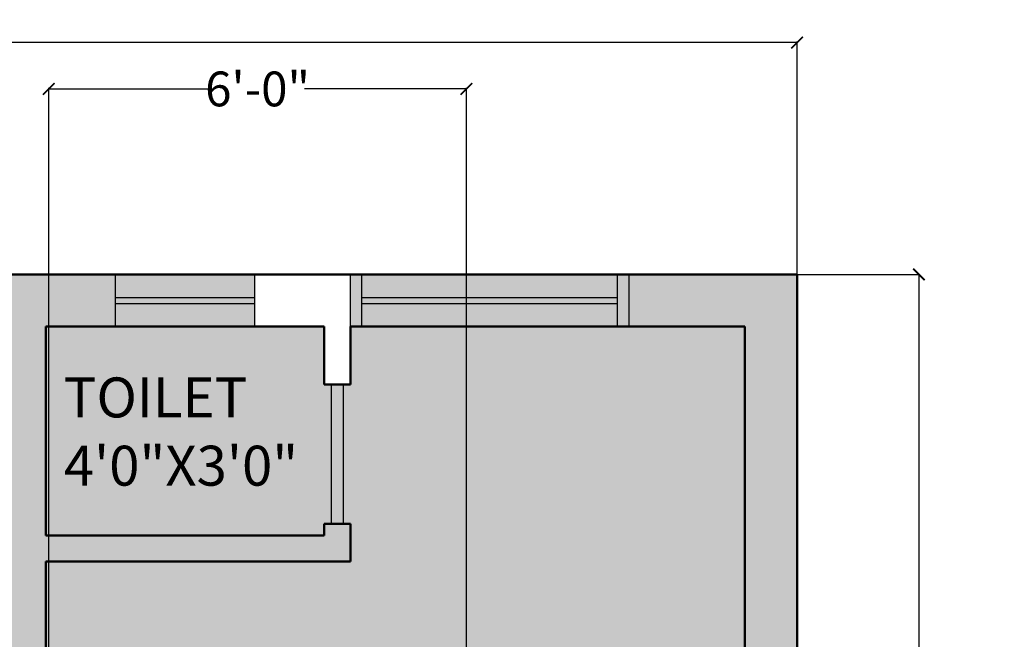
# Model space of a CAD drawing. Units: inches. Extents: x 528 to 2620, y -1066 to 798.
# Tile 34 of 41: x 1211 to 1381, y 656 to 763. Entities that reach past the tile are written whole.
import ezdxf

# ---------------------------------------------------------------- set-up
doc = ezdxf.new("R2010")
doc.units = ezdxf.units.IN
doc.header["$MEASUREMENT"] = 0
for name, color, linetype, lineweight in [('A-ANNO-DIMS', 2, 'Continuous', 18), ('A-AREA-IDEN', 7, 'Continuous', 18), ('A-Door', 2, 'Continuous', 25), ('A-GLAZ', 3, 'Continuous', 25), ('A-WALL', 7, 'Continuous', 50), ('A-WALL-PATT', 8, 'Continuous', 13)]:
    doc.layers.add(name, color=color, linetype=linetype, lineweight=lineweight)
doc.styles.get("Standard").update_dxf_attribs({"font": 'arial.ttf'})
doc.dimstyles.get("Standard").update_dxf_attribs({"dimtxt": 6, "dimasz": 2, "dimexe": 0.18, "dimexo": 0.0625, "dimgap": 0.09, "dimtad": 0, "dimtih": 1, "dimtoh": 1, "dimdec": 1, "dimzin": 0, "dimdsep": 46, "dimlunit": 3, "dimtxsty": 'Standard', "dimblk": 'ARCHTICK', "dimcen": 0.09, "dimadec": 0, "dimazin": 0, "dimtfac": 1, "dimtdec": 1, "dimtofl": 0, "dimtmove": 0, "dimatfit": 3, "dimfxl": 1, "dimtolj": 1, "dimtzin": 0, "dimarcsym": 0})

# ---------------------------------------------------------------- blocks, each defined once
blk = doc.blocks.new('_ArchTick')
at = {"color": 0, "linetype": 'ByBlock', "const_width": 0.15}
blk.add_lwpolyline([(-0.5, -0.5), (0.5, 0.5)], dxfattribs=at)
blk = doc.blocks.new('*D17')
at = {"layer": 'A-ANNO-DIMS', "color": 0, "lineweight": -2, "transparency": 16777216}
for p, q in [((1345.06, 718.92), (1366.18, 718.92)), ((1366, 718.92), (1366, 497.08)), ((1366, 268.92), (1366, 490.77)), ((1345.06, 268.92), (1366.18, 268.92))]:
    blk.add_line(p, q, dxfattribs=at)
at = {"layer": 'Defpoints', "color": 0, "transparency": 16777216}
for p in [(1345, 718.92), (1345, 268.92), (1366, 268.92)]:
    blk.add_point(p, dxfattribs=at)
at = {"layer": 'A-ANNO-DIMS', "color": 0, "lineweight": -2, "transparency": 16777216, "xscale": 2, "yscale": 2, "zscale": 2}
for p, rotation in [((1366, 718.92), 90), ((1366, 268.92), 270)]:
    blk.add_blockref('_ArchTick', p, dxfattribs=dict(at, rotation=rotation))
at = {"layer": 'A-ANNO-DIMS', "color": 0, "transparency": 16777216, "insert": (1366, 493.92), "char_height": 6, "attachment_point": 5}
blk.add_mtext('\\A1;37\'-6.0"', dxfattribs=at)
blk = doc.blocks.new('*D18')
at = {"layer": 'A-ANNO-DIMS', "color": 0, "lineweight": -2, "transparency": 16777216}
for p, q in [((1057, 718.98), (1057, 759.11)), ((1057, 758.93), (1195.76, 758.93)), ((1345, 758.93), (1206.23, 758.93)), ((1345, 718.98), (1345, 759.11))]:
    blk.add_line(p, q, dxfattribs=at)
at = {"layer": 'Defpoints', "color": 0, "transparency": 16777216}
for p in [(1345, 758.93), (1057, 718.92), (1345, 718.92)]:
    blk.add_point(p, dxfattribs=at)
at = {"layer": 'A-ANNO-DIMS', "color": 0, "lineweight": -2, "transparency": 16777216, "xscale": 2, "yscale": 2, "zscale": 2, "rotation": 180}
blk.add_blockref('_ArchTick', (1057, 758.93), dxfattribs=at)
at = {"layer": 'A-ANNO-DIMS', "color": 0, "lineweight": -2, "transparency": 16777216, "xscale": 2, "yscale": 2, "zscale": 2}
blk.add_blockref('_ArchTick', (1345, 758.93), dxfattribs=at)
at = {"layer": 'A-ANNO-DIMS', "color": 0, "transparency": 16777216, "insert": (1201, 758.93), "char_height": 6, "attachment_point": 5}
blk.add_mtext("\\A1;24'", dxfattribs=at)
blk = doc.blocks.new('WIN-1200')
for p, q in [((677.56, 718.92), (725.56, 718.92)), ((677.56, 709.92), (677.56, 718.92)), ((679.56, 709.92), (679.56, 718.92)), ((723.56, 718.92), (723.56, 709.92)), ((725.56, 718.92), (725.56, 709.92)), ((679.56, 714.92), (723.56, 714.92)), ((679.56, 713.92), (723.56, 713.92)), ((725.56, 709.92), (677.56, 709.92))]:
    blk.add_line(p, q)
blk = doc.blocks.new('WIN-600')
for p, q in [((790.56, 714.92), (814.56, 714.92)), ((790.56, 713.92), (814.56, 713.92))]:
    blk.add_line(p, q)
blk.add_lwpolyline([(790.56, 718.92), (814.56, 718.92), (814.56, 709.92), (790.56, 709.92)], close=True)
blk = doc.blocks.new('*D68')
at = {"layer": 'A-ANNO-DIMS', "color": 0, "lineweight": -2, "transparency": 16777216}
for p, q in [((1216, 400.48), (1216, 751.1)), ((1216, 750.92), (1243.92, 750.92)), ((1288, 750.92), (1260.08, 750.92)), ((1288, 395.98), (1288, 751.1))]:
    blk.add_line(p, q, dxfattribs=at)
at = {"layer": 'Defpoints', "color": 0, "transparency": 16777216}
for p in [(1288, 750.92), (1216, 400.42), (1288, 395.92)]:
    blk.add_point(p, dxfattribs=at)
at = {"layer": 'A-ANNO-DIMS', "color": 0, "lineweight": -2, "transparency": 16777216, "xscale": 2, "yscale": 2, "zscale": 2, "rotation": 180}
blk.add_blockref('_ArchTick', (1216, 750.92), dxfattribs=at)
at = {"layer": 'A-ANNO-DIMS', "color": 0, "lineweight": -2, "transparency": 16777216, "xscale": 2, "yscale": 2, "zscale": 2}
blk.add_blockref('_ArchTick', (1288, 750.92), dxfattribs=at)
at = {"layer": 'A-ANNO-DIMS', "color": 0, "transparency": 16777216, "insert": (1252, 750.92), "char_height": 6, "attachment_point": 5}
blk.add_mtext('\\A1;6\'-0"', dxfattribs=at)

msp = doc.modelspace()

# ---------------------------------------------------------------- hatches: boundary and pattern name
at = {"layer": 'A-Door', "transparency": 33554521}
h = msp.add_hatch(color=256, dxfattribs=at)
h.dxf.hatch_style = 1
h.paths.add_polyline_path([(1266.75, 699.92), (1264.75, 699.92), (1264.75, 675.92), (1266.75, 675.92)])
at = {"layer": 'A-WALL-PATT', "transparency": 33554521}
h = msp.add_hatch(color=256, dxfattribs=at)
h.dxf.hatch_style = 1
h.paths.add_polyline_path([(1066, 709.92), (1114.5, 709.92), (1114.5, 718.92), (1057, 718.92), (1057, 667.92), (1066, 667.92)])
h.paths.add_polyline_path([(1227.5, 718.92), (1162.5, 718.92), (1162.5, 709.92), (1211, 709.92), (1211, 577.92), (1205.42, 577.92), (1205.5, 573.42), (1211, 573.42), (1211, 567.42), (1215.5, 567.42), (1215.5, 669.42), (1268, 669.42), (1268, 675.92), (1263.5, 675.92), (1263.5, 673.92), (1215.5, 673.92), (1215.5, 709.92), (1227.5, 709.92)])
h.paths.add_polyline_path([(1345, 718.92), (1316, 718.92), (1316, 709.92), (1336, 709.92), (1336, 641.67), (1345, 641.67)])
h.paths.add_polyline_path([(1066, 619.92), (1057, 619.92), (1057, 561.42), (1066, 561.42), (1066, 573.42), (1161, 573.42), (1161, 569.42), (1165.5, 569.42), (1165.5, 577.92), (1066, 577.92)])
h.paths.add_polyline_path([(1216, 391.42), (1216, 400.42), (1207, 400.42), (1201, 400.42), (1201, 397.42), (1201, 391.42), (1207, 391.42), (1207, 268.92), (1252, 268.92), (1252, 277.92), (1216, 277.92), (1216, 359.77)])
h.paths.add_polyline_path([(1345, 395.92), (1336, 395.92), (1288, 395.92), (1288, 391.42), (1336, 391.42), (1336, 277.92), (1300, 277.92), (1300, 268.92), (1345, 268.92)])
h.paths.add_polyline_path([(1345, 593.67), (1336, 593.67), (1336, 525.42), (1215.5, 525.42), (1215.5, 527.17), (1211, 527.17), (1211, 520.92), (1336, 520.92), (1336, 443.92), (1345, 443.92)])
h.paths.add_polyline_path([(1066, 520.92), (1165.5, 520.92), (1165.5, 545.42), (1161, 545.42), (1161, 525.42), (1066, 525.42), (1066, 537.42), (1057, 537.42), (1057, 484.67), (1066, 484.67)])
h.paths.add_polyline_path([(1066, 436.67), (1057, 436.67), (1057, 391.42), (1085.5, 391.42), (1085.5, 400.42), (1066, 400.42)])
h.paths.add_polyline_path([(1153, 397.42), (1153, 400.42), (1133.5, 400.42), (1133.5, 391.42), (1153, 391.42)])
at = {"layer": 'A-WALL-PATT', "transparency": 33554681}
h = msp.add_hatch(color=256, dxfattribs=at)
h.dxf.hatch_style = 1
h.paths.add_polyline_path([(1062, 665.92), (1061, 665.92), (1061, 621.92), (1062, 621.92)])
h.paths.add_polyline_path([(1066, 667.92), (1057, 667.92), (1057, 665.92), (1066, 665.92)])
h.paths.add_polyline_path([(1066, 621.92), (1057, 621.92), (1057, 619.92), (1066, 619.92)])
h.paths.add_polyline_path([(1160.5, 714.92), (1116.5, 714.92), (1116.5, 713.92), (1160.5, 713.92)])
h.paths.add_polyline_path([(1162.5, 718.92), (1160.5, 718.92), (1160.5, 709.92), (1162.5, 709.92)])
h.paths.add_polyline_path([(1116.5, 718.92), (1114.5, 718.92), (1114.5, 709.92), (1116.5, 709.92)])
h.paths.add_polyline_path([(1251.5, 714.92), (1227.5, 714.92), (1227.5, 713.92), (1251.5, 713.92)])
h.paths.add_polyline_path([(1314, 714.92), (1270, 714.92), (1270, 713.92), (1314, 713.92)])
h.paths.add_polyline_path([(1316, 718.92), (1314, 718.92), (1314, 709.92), (1316, 709.92)])
h.paths.add_polyline_path([(1270, 718.92), (1268, 718.92), (1268, 709.92), (1270, 709.92)])
h.paths.add_polyline_path([(1087.5, 400.42), (1085.5, 400.42), (1085.5, 391.42), (1087.5, 391.42)])
h.paths.add_polyline_path([(1131.5, 396.42), (1087.5, 396.42), (1087.5, 395.42), (1131.5, 395.42)])
h.paths.add_polyline_path([(1133.5, 400.42), (1131.5, 400.42), (1131.5, 391.42), (1133.5, 391.42)])
h.paths.add_polyline_path([(1066, 438.67), (1057, 438.67), (1057, 436.67), (1066, 436.67)])
h.paths.add_polyline_path([(1066, 484.67), (1057, 484.67), (1057, 482.67), (1066, 482.67)])
h.paths.add_polyline_path([(1062, 482.67), (1061, 482.67), (1061, 438.67), (1062, 438.67)])
h = msp.add_hatch(color=256, dxfattribs=at)
h.dxf.hatch_style = 1
h.paths.add_polyline_path([(1066, 665.92), (1062, 665.92), (1062, 621.92), (1066, 621.92)])
h.paths.add_polyline_path([(1061, 665.92), (1057, 665.92), (1057, 621.92), (1061, 621.92)])
h.paths.add_polyline_path([(1160.5, 713.92), (1116.5, 713.92), (1116.5, 709.92), (1160.5, 709.92)])
h.paths.add_polyline_path([(1160.5, 718.92), (1116.5, 718.92), (1116.5, 714.92), (1160.5, 714.92)])
h.paths.add_polyline_path([(1251.5, 713.92), (1227.5, 713.92), (1227.5, 709.92), (1251.5, 709.92)])
h.paths.add_polyline_path([(1251.5, 718.92), (1227.5, 718.92), (1227.5, 714.92), (1251.5, 714.92)])
h.paths.add_polyline_path([(1314, 713.92), (1270, 713.92), (1270, 709.92), (1314, 709.92)])
h.paths.add_polyline_path([(1314, 718.92), (1270, 718.92), (1270, 714.92), (1314, 714.92)])
h.paths.add_polyline_path([(1345, 639.67), (1341, 639.67), (1341, 595.67), (1345, 595.67)])
h.paths.add_polyline_path([(1340, 639.67), (1336, 639.67), (1336, 595.67), (1340, 595.67)])
h.paths.add_polyline_path([(1345, 441.92), (1341, 441.92), (1341, 397.92), (1345, 397.92)])
h.paths.add_polyline_path([(1340, 441.92), (1336, 441.92), (1336, 397.92), (1340, 397.92)])
h.paths.add_polyline_path([(1298, 272.92), (1254, 272.92), (1254, 268.92), (1298, 268.92)])
h.paths.add_polyline_path([(1298, 277.92), (1254, 277.92), (1254, 273.92), (1298, 273.92)])
h.paths.add_polyline_path([(1131.5, 395.42), (1087.5, 395.42), (1087.5, 391.42), (1131.5, 391.42)])
h.paths.add_polyline_path([(1131.5, 400.42), (1087.5, 400.42), (1087.5, 396.42), (1131.5, 396.42)])
h.paths.add_polyline_path([(1066, 482.67), (1062, 482.67), (1062, 438.67), (1066, 438.67)])
h.paths.add_polyline_path([(1061, 482.67), (1057, 482.67), (1057, 438.67), (1061, 438.67)])
h.paths.add_polyline_path([(1066, 561.42), (1062, 561.42), (1062, 537.42), (1066, 537.42)])
h.paths.add_polyline_path([(1061, 561.42), (1057, 561.42), (1057, 537.42), (1061, 537.42)])
at = {"layer": 'A-WALL-PATT', "transparency": 33554536}
h = msp.add_hatch(color=256, dxfattribs=at)
h.dxf.hatch_style = 1
h.paths.add_polyline_path([(1336, 709.92), (1268, 709.92), (1268, 699.92), (1266.75, 699.92), (1266.75, 675.92), (1268, 675.92), (1268, 669.42), (1215.5, 669.42), (1215.5, 567.17), (1217, 567.17), (1257, 567.17), (1257, 565.42), (1256.96, 565.42, -0.401453), (1217, 527.17), (1215.5, 527.17), (1215.5, 525.42), (1336, 525.42)], flags=17)
h.paths.add_polyline_path([(1285.03, 635.93), (1285.23, 636.13), (1285.67, 636.26), (1286.21, 636.02), (1286.98, 636.08), (1332.98, 636.08), (1333.36, 636.22), (1333.82, 636.08), (1334.11, 635.71), (1334.11, 635.3), (1333.91, 634.86), (1333.82, 634.83), (1333.82, 592.74), (1333.97, 592.6), (1334.11, 592.29), (1334.11, 591.88), (1333.82, 591.51), (1333.36, 591.37), (1332.98, 591.51), (1332.64, 591.79), (1332.64, 591.51), (1286.98, 591.51), (1286.17, 591.67), (1286.07, 591.57), (1285.68, 591.37), (1285.23, 591.51), (1285.03, 591.71), (1284.83, 592.1), (1284.98, 592.54), (1285.13, 592.69), (1285.13, 634.95), (1284.98, 635.1), (1284.83, 635.54)], flags=16)
h.paths.add_polyline_path([(1285.03, 635.93), (1285.23, 636.13), (1285.67, 636.26), (1286.21, 636.02), (1286.98, 636.08), (1332.98, 636.08), (1333.36, 636.22), (1333.82, 636.08), (1334.11, 635.71), (1334.11, 635.3), (1333.97, 634.99), (1333.82, 634.85), (1333.82, 592.74), (1333.97, 592.6), (1334.11, 592.29), (1334.11, 591.88), (1333.82, 591.51), (1333.36, 591.37), (1332.98, 591.51), (1332.64, 591.79), (1332.64, 592.25), (1332.64, 635.35), (1332.64, 635.8), (1332.98, 636.08), (1312.23, 636.08), (1311.1, 635.48), (1310.63, 635.48), (1310.43, 635.23), (1309.94, 635.1), (1309.7, 634.99), (1309.06, 634.76), (1308.71, 634.61), (1308.32, 634.61), (1307.75, 634.36), (1307.11, 634.27), (1307.01, 634.11), (1306.77, 634.02), (1307.25, 633.28), (1306.87, 633.04), (1306.77, 632.88), (1306.37, 632.64), (1306.03, 632.55), (1305.54, 632.41), (1315.47, 618.49), (1316.32, 619.39), (1312.77, 622.86), (1319.62, 630.11), (1320.07, 629.68), (1320.11, 630), (1320.28, 630.6), (1320.53, 631.18), (1320.53, 632.01), (1320.26, 632.55), (1320.11, 633.13), (1320.06, 633.73), (1320.63, 634.02), (1321.22, 634.16), (1321.86, 634.11), (1322.45, 633.91), (1322.99, 633.62), (1324.1, 633.62), (1324.64, 633.91), (1325.23, 634.07), (1325.87, 634.07), (1326.43, 633.91), (1326.98, 633.62), (1328.35, 633.62), (1328.9, 633.91), (1329.49, 634.11), (1330.1, 634.16), (1330.69, 634.02), (1331.28, 633.73), (1331.23, 633.13), (1331.09, 632.55), (1330.79, 632.01), (1330.79, 631.18), (1331.04, 630.6), (1331.23, 630), (1331.28, 629.41), (1331.19, 628.79), (1331.04, 628.18), (1330.79, 627.6), (1330.79, 626.77), (1331.04, 626.19), (1331.23, 625.59), (1331.28, 625.01), (1331.19, 624.38), (1331.04, 623.78), (1330.79, 623.24), (1330.79, 622.37), (1331.04, 621.83), (1331.23, 621.25), (1331.28, 620.6), (1331.19, 619.97), (1331.04, 619.37), (1330.79, 618.83), (1330.79, 617.96), (1331.09, 617.42), (1331.23, 616.88), (1331.28, 616.23), (1331.28, 615.52), (1330.69, 615.27), (1330.1, 615.12), (1329.49, 615.12), (1328.9, 615.32), (1328.35, 615.65), (1326.98, 615.65), (1326.43, 615.32), (1325.87, 615.16), (1325.23, 615.16), (1324.64, 615.32), (1324.1, 615.65), (1323.24, 615.65), (1324.93, 614.04), (1322.98, 611.98), (1324.1, 611.98), (1324.64, 612.27), (1325.28, 612.43), (1325.87, 612.43), (1326.48, 612.27), (1327.03, 611.98), (1328.35, 611.98), (1328.9, 612.27), (1329.49, 612.48), (1330.1, 612.52), (1330.74, 612.39), (1331.28, 612.07), (1331.28, 611.36), (1331.28, 610.75), (1331.09, 610.17), (1330.79, 609.63), (1330.79, 608.81), (1331.09, 608.22), (1331.23, 607.62), (1331.28, 606.99), (1331.23, 606.41), (1331.09, 605.81), (1330.79, 605.22), (1330.79, 604.4), (1331.09, 603.81), (1331.23, 603.21), (1331.28, 602.63), (1331.23, 602), (1331.09, 601.4), (1330.79, 600.86), (1330.79, 599.99), (1331.09, 599.45), (1331.23, 598.87), (1331.28, 598.22), (1331.23, 597.59), (1331.09, 596.99), (1330.79, 596.45), (1330.79, 595.58), (1331.09, 595.04), (1331.28, 594.51), (1331.28, 593.86), (1330.74, 593.61), (1330.1, 593.48), (1329.49, 593.48), (1328.9, 593.68), (1328.35, 594.01), (1327.03, 594.01), (1326.48, 593.68), (1325.87, 593.52), (1325.28, 593.52), (1324.64, 593.68), (1324.1, 594.01), (1323.04, 594.01), (1322.5, 593.68), (1321.91, 593.48), (1321.27, 593.48), (1320.63, 593.61), (1320.11, 593.86), (1320.11, 594.51), (1320.28, 595.04), (1320.58, 595.58), (1320.58, 596.45), (1320.28, 596.99), (1320.16, 597.59), (1320.1, 598.01), (1319.62, 597.55), (1315.66, 601.73), (1312.23, 591.57), (1311.74, 591.66), (1311.59, 591.91), (1310.78, 592.4), (1309.55, 592.89), (1308.96, 592.89), (1308.71, 593.03), (1308.56, 593.14), (1307.75, 593.52), (1306.77, 593.61), (1307.25, 594.36), (1306.87, 594.6), (1306.37, 594.84), (1306.03, 595.09), (1305.54, 595.24), (1315.46, 609.35), (1310.93, 613.71), (1315.47, 618.49), (1305.54, 632.41), (1306.03, 632.55), (1306.37, 632.64), (1306.77, 632.88), (1306.87, 633.04), (1307.25, 633.28), (1306.77, 634.02), (1307.01, 634.11), (1307.11, 634.27), (1307.75, 634.36), (1308.32, 634.61), (1308.71, 634.61), (1309.06, 634.76), (1309.7, 634.99), (1309.94, 635.1), (1310.43, 635.23), (1310.63, 635.48), (1311.1, 635.48), (1312.23, 636.08), (1286.98, 636.08), (1286.22, 636.02), (1286.41, 635.44), (1286.21, 635.05), (1286.02, 634.85), (1285.87, 634.81), (1285.87, 592.84), (1286.15, 592.73), (1286.41, 592.19), (1286.23, 591.66), (1286.17, 591.67), (1286.07, 591.57), (1285.68, 591.37), (1285.23, 591.51), (1285.03, 591.71), (1284.83, 592.1), (1284.98, 592.54), (1285.13, 592.69), (1285.13, 634.95), (1284.98, 635.1), (1284.83, 635.54)], flags=0)
h.paths.add_polyline_path([(1322.5, 653.6), (1333.65, 653.6), (1333.65, 637.99), (1322.5, 637.99)], flags=16)
h.paths.add_polyline_path([(1323.62, 652.48), (1332.53, 652.48), (1332.53, 639.11), (1323.62, 639.11)], flags=0)
edge = h.paths.add_edge_path(flags=0)
edge.add_ellipse((1328.07, 645.79), major_axis=(2.24, 2.24), ratio=1, start_angle=405, end_angle=495, ccw=False)
edge.add_ellipse((1328.07, 645.79), major_axis=(2.24, 2.24), ratio=1, start_angle=675, end_angle=765, ccw=False)
edge.add_ellipse((1328.07, 645.79), major_axis=(2.24, 2.24), ratio=1, start_angle=585, end_angle=675, ccw=False)
edge.add_ellipse((1328.07, 645.79), major_axis=(2.24, 2.24), ratio=1, start_angle=495, end_angle=585, ccw=False)
h.paths.add_polyline_path([(1320.58, 628.39), (1320.33, 628.01), (1320.61, 628.55)], flags=0)
h.paths.add_polyline_path([(1317.89, 604.89), (1318.78, 604.64), (1319.76, 604.28), (1318.88, 604.53)], flags=0)
h.paths.add_polyline_path([(1320.33, 599.65), (1320.58, 599.25), (1320.58, 599.16)], flags=0)
h.paths.add_polyline_path([(1322.5, 589.6), (1333.65, 589.6), (1333.65, 573.99), (1322.5, 573.99)], flags=16)
h.paths.add_polyline_path([(1323.62, 588.48), (1332.53, 588.48), (1332.53, 575.11), (1323.62, 575.11)], flags=0)
edge = h.paths.add_edge_path(flags=0)
edge.add_ellipse((1328.07, 581.8), major_axis=(-2.24, 2.24), ratio=1, start_angle=-45, end_angle=45, ccw=False)
edge.add_ellipse((1328.07, 581.8), major_axis=(-2.24, 2.24), ratio=1, start_angle=-135, end_angle=-45, ccw=False)
edge.add_ellipse((1328.07, 581.8), major_axis=(-2.24, 2.24), ratio=1, start_angle=135, end_angle=-135, ccw=False)
edge.add_ellipse((1328.07, 581.8), major_axis=(-2.24, 2.24), ratio=1, start_angle=45, end_angle=135, ccw=False)
h.paths.add_polyline_path([(1264.75, 699.92), (1263.5, 699.92), (1263.5, 709.92), (1215.5, 709.92), (1215.5, 673.92), (1263.5, 673.92), (1263.5, 675.92), (1264.75, 675.92)], flags=16)
h.paths.add_polyline_path([(1162.19, 569.42), (1161, 569.42), (1161, 573.42), (1066, 573.42), (1066, 525.42), (1161, 525.42), (1161, 545.42), (1162.19, 545.42)])
h.paths.add_polyline_path([(1256.96, 565.42), (1257, 565.42), (1257, 567.17), (1217, 567.17), (1215.5, 567.17), (1215.5, 567.42), (1211, 567.42), (1211, 573.42), (1205.5, 573.42), (1205.42, 577.92), (1211, 577.92), (1211, 709.92), (1066, 709.92), (1066, 577.92), (1165.5, 577.92), (1165.5, 569.42), (1164.19, 569.42), (1164.19, 545.42), (1165.5, 545.42), (1165.5, 520.92), (1153, 520.92), (1153, 484.92), (1102, 484.92), (1102, 436.42), (1153, 436.42), (1153, 400.42), (1153, 391.42), (1201, 391.42), (1201, 400.42), (1207, 400.42), (1216, 400.42), (1216, 391.42), (1216, 277.92), (1336, 277.92), (1336, 391.42), (1288, 391.42), (1288, 395.92), (1336, 395.92), (1336, 443.92), (1336, 520.92), (1211, 520.92), (1211, 527.17), (1215.5, 527.17), (1217, 527.17, 0.401453)])
h.paths.add_polyline_path([(1167.25, 579.42), (1165.5, 579.42), (1165.5, 619.42), (1167.25, 619.42)], flags=16)
h.paths.add_polyline_path([(1227.97, 501.56), (1236.36, 502.03), (1236.36, 492.55), (1227.97, 493.02, -0.254069)], flags=16)
h.paths.add_polyline_path([(1243.34, 515.69, -0.254069), (1251.88, 515.69), (1252.35, 507.3), (1242.87, 507.3)], flags=16)
h.paths.add_polyline_path([(1239.18, 504.68), (1256.03, 504.68), (1256.03, 479.42), (1239.18, 479.42)], flags=16)
h.paths.add_polyline_path([(1227.97, 489.6), (1236.36, 490.07), (1236.36, 480.59), (1227.97, 481.06, -0.254069)], flags=16)
h.paths.add_polyline_path([(1197.2, 624.04), (1197.2, 639.64), (1208.35, 639.64), (1208.35, 624.04)], flags=16)
h.paths.add_polyline_path([(1198.32, 625.15), (1198.32, 638.53), (1207.23, 638.53), (1207.23, 625.15)], flags=0)
h.paths.add_polyline_path([(1258.85, 502.03), (1267.25, 501.56, -0.254069), (1267.25, 493.02), (1258.85, 492.55)], flags=16)
h.paths.add_polyline_path([(1271.59, 519.66), (1333.67, 519.66), (1333.67, 451.59), (1319.09, 451.59), (1319.09, 505.07), (1288.09, 505.07), (1284.45, 505.07, -0.883215), (1270.68, 514.19), (1270.68, 518.75, -0.414214)], flags=16)
h.paths.add_polyline_path([(1331.85, 517.83), (1331.85, 453.42), (1328.2, 453.42), (1328.2, 505.07), (1298.42, 505.07), (1298.42, 514.19), (1288.09, 514.19), (1288.09, 517.83)], flags=0)
h.paths.add_polyline_path([(1242.87, 476.8), (1252.35, 476.8), (1251.88, 468.41, -0.254069), (1243.34, 468.41)], flags=16)
h.paths.add_polyline_path([(1258.85, 490.07), (1267.25, 489.6, -0.254069), (1267.25, 481.06), (1258.85, 480.59)], flags=16)
h.paths.add_polyline_path([(1161.68, 641.55), (1160.87, 641.72), (1160.77, 641.62), (1160.38, 641.41), (1159.93, 641.55), (1159.73, 641.75), (1159.53, 642.14), (1159.68, 642.58), (1159.83, 642.73), (1159.83, 684.99), (1159.68, 685.14), (1159.53, 685.58), (1159.73, 685.97), (1159.93, 686.17), (1160.37, 686.31), (1160.91, 686.06), (1161.68, 686.13), (1207.68, 686.13), (1208.06, 686.27), (1208.52, 686.13), (1208.81, 685.76), (1208.81, 685.34), (1208.61, 684.9), (1208.52, 684.87), (1208.52, 642.78), (1208.67, 642.65), (1208.88, 642.2), (1208.72, 641.8), (1208.52, 641.55), (1208.06, 641.41), (1207.68, 641.55), (1207.34, 641.83), (1207.34, 641.55)], flags=16)
h.paths.add_polyline_path([(1186.93, 641.62), (1186.44, 641.71), (1186.29, 641.95), (1185.48, 642.45), (1184.25, 642.94), (1183.66, 642.94), (1183.41, 643.07), (1183.26, 643.18), (1182.45, 643.57), (1181.47, 643.65), (1181.95, 644.4), (1181.57, 644.64), (1181.07, 644.89), (1180.73, 645.13), (1180.24, 645.29), (1190.16, 659.4), (1185.63, 663.75), (1190.17, 668.54), (1180.24, 682.46), (1180.73, 682.59), (1181.07, 682.68), (1181.47, 682.93), (1181.57, 683.08), (1181.95, 683.33), (1181.47, 684.07), (1181.71, 684.16), (1181.81, 684.31), (1182.45, 684.4), (1183.02, 684.65), (1183.41, 684.65), (1183.76, 684.81), (1184.4, 685.03), (1184.64, 685.14), (1185.13, 685.28), (1185.33, 685.52), (1185.8, 685.52), (1186.93, 686.13), (1161.68, 686.13), (1160.92, 686.06), (1161.11, 685.49), (1160.91, 685.1), (1160.72, 684.9), (1160.57, 684.85), (1160.57, 642.88), (1160.85, 642.77), (1161.11, 642.23), (1160.93, 641.7), (1160.87, 641.72), (1160.77, 641.62), (1160.38, 641.41), (1159.93, 641.55), (1159.73, 641.75), (1159.53, 642.14), (1159.68, 642.58), (1159.83, 642.73), (1159.83, 684.99), (1159.68, 685.14), (1159.53, 685.58), (1159.73, 685.97), (1159.93, 686.17), (1160.37, 686.31), (1160.91, 686.06), (1161.68, 686.13), (1207.68, 686.13), (1208.06, 686.27), (1208.52, 686.13), (1208.81, 685.76), (1208.81, 685.34), (1208.67, 685.03), (1208.52, 684.9), (1208.52, 642.78), (1208.67, 642.65), (1208.88, 642.2), (1208.72, 641.8), (1208.52, 641.55), (1208.06, 641.41), (1207.68, 641.55), (1207.34, 641.83), (1207.34, 642.29), (1207.34, 685.39), (1207.34, 685.85), (1207.68, 686.13), (1186.93, 686.13), (1185.8, 685.52), (1185.33, 685.52), (1185.13, 685.28), (1184.64, 685.14), (1184.4, 685.03), (1183.76, 684.81), (1183.41, 684.65), (1183.02, 684.65), (1182.45, 684.4), (1181.81, 684.31), (1181.71, 684.16), (1181.47, 684.07), (1181.95, 683.33), (1181.57, 683.08), (1181.47, 682.93), (1181.07, 682.68), (1180.73, 682.59), (1180.24, 682.46), (1190.17, 668.54), (1191.02, 669.43), (1187.47, 672.9), (1194.32, 680.15), (1194.77, 679.72), (1194.81, 680.04), (1194.98, 680.65), (1195.23, 681.23), (1195.23, 682.05), (1194.96, 682.59), (1194.81, 683.17), (1194.76, 683.78), (1195.33, 684.07), (1195.92, 684.2), (1196.56, 684.16), (1197.15, 683.96), (1197.69, 683.67), (1198.8, 683.67), (1199.34, 683.96), (1199.93, 684.11), (1200.57, 684.11), (1201.13, 683.96), (1201.68, 683.67), (1203.05, 683.67), (1203.6, 683.96), (1204.19, 684.16), (1204.8, 684.2), (1205.39, 684.07), (1205.98, 683.78), (1205.93, 683.17), (1205.79, 682.59), (1205.49, 682.05), (1205.49, 681.23), (1205.74, 680.65), (1205.93, 680.04), (1205.98, 679.46), (1205.89, 678.83), (1205.74, 678.23), (1205.49, 677.65), (1205.49, 676.82), (1205.74, 676.24), (1205.93, 675.63), (1205.98, 675.05), (1205.89, 674.42), (1205.74, 673.82), (1205.49, 673.28), (1205.49, 672.41), (1205.74, 671.87), (1205.93, 671.29), (1205.98, 670.64), (1205.89, 670.02), (1205.74, 669.41), (1205.49, 668.87), (1205.49, 668), (1205.79, 667.46), (1205.93, 666.93), (1205.98, 666.28), (1205.98, 665.56), (1205.39, 665.32), (1204.8, 665.16), (1204.19, 665.16), (1203.6, 665.36), (1203.05, 665.7), (1201.68, 665.7), (1201.13, 665.36), (1200.57, 665.2), (1199.93, 665.2), (1199.34, 665.36), (1198.8, 665.7), (1197.94, 665.7), (1199.63, 664.09), (1197.68, 662.03), (1198.8, 662.03), (1199.34, 662.32), (1199.98, 662.47), (1200.57, 662.47), (1201.18, 662.32), (1201.73, 662.03), (1203.05, 662.03), (1203.6, 662.32), (1204.19, 662.52), (1204.8, 662.56), (1205.44, 662.43), (1205.98, 662.12), (1205.98, 661.4), (1205.98, 660.8), (1205.79, 660.21), (1205.49, 659.68), (1205.49, 658.85), (1205.79, 658.27), (1205.93, 657.66), (1205.98, 657.04), (1205.93, 656.45), (1205.79, 655.85), (1205.49, 655.27), (1205.49, 654.44), (1205.79, 653.86), (1205.93, 653.25), (1205.98, 652.67), (1205.93, 652.05), (1205.79, 651.44), (1205.49, 650.91), (1205.49, 650.03), (1205.79, 649.5), (1205.93, 648.91), (1205.98, 648.26), (1205.93, 647.64), (1205.79, 647.03), (1205.49, 646.5), (1205.49, 645.62), (1205.79, 645.09), (1205.98, 644.55), (1205.98, 643.9), (1205.44, 643.65), (1204.8, 643.52), (1204.19, 643.52), (1203.6, 643.72), (1203.05, 644.06), (1201.73, 644.06), (1201.18, 643.72), (1200.57, 643.57), (1199.98, 643.57), (1199.34, 643.72), (1198.8, 644.06), (1197.74, 644.06), (1197.2, 643.72), (1196.61, 643.52), (1195.97, 643.52), (1195.33, 643.65), (1194.81, 643.9), (1194.81, 644.55), (1194.98, 645.09), (1195.28, 645.62), (1195.28, 646.5), (1194.98, 647.03), (1194.86, 647.64), (1194.8, 648.06), (1194.32, 647.59), (1190.36, 651.77)], flags=16)
h.paths.add_polyline_path([(1195.28, 649.2), (1195.03, 649.7), (1195.28, 649.29)], flags=0)
h.paths.add_polyline_path([(1194.46, 654.33), (1193.58, 654.58), (1192.59, 654.93), (1193.48, 654.69)], flags=0)
h.paths.add_polyline_path([(1195.28, 678.43), (1195.03, 678.05), (1195.31, 678.59)], flags=0)
h.paths.add_polyline_path([(1197.2, 688.04), (1197.2, 703.64), (1208.35, 703.64), (1208.35, 688.04)], flags=16)
h.paths.add_polyline_path([(1198.32, 689.15), (1198.32, 702.53), (1207.23, 702.53), (1207.23, 689.15)], flags=0)
h.paths.add_polyline_path([(1217.1, 329.02), (1230.65, 329.02), (1230.65, 315.47), (1217.1, 315.47)], flags=16)
h.paths.add_polyline_path([(1223.87, 322.24), (1227.26, 322.24), (1227.26, 321.32, -0.414214), (1229.73, 318.86, -1), (1224.8, 318.86), (1223.87, 318.86)], flags=0)
h.paths.add_polyline_path([(1222.11, 325.63, -1), (1218.86, 325.63, -1)], flags=0)
h.paths.add_polyline_path([(1228.25, 325.63, -1), (1226.28, 325.63, -1)], flags=0)
h.paths.add_polyline_path([(1221.53, 318.86, -1), (1219.44, 318.86, -1)], flags=0)
h.paths.add_polyline_path([(1299.15, 293.73), (1299.15, 278.54), (1271.23, 278.54), (1271.23, 293.73)], flags=16)
h.paths.add_polyline_path([(1259.69, 292.21), (1270.62, 292.21, -1), (1270.62, 291.6), (1259.69, 291.6, -1)], flags=16)
h.paths.add_polyline_path([(1259.69, 291.3), (1270.62, 291.3, -1), (1270.62, 290.69), (1259.69, 290.69, -1)], flags=16)
h.paths.add_polyline_path([(1259.69, 290.39), (1270.62, 290.39, -1), (1270.62, 289.78), (1259.69, 289.78, -1)], flags=16)
h.paths.add_polyline_path([(1259.69, 289.48), (1270.62, 289.48, -1), (1270.62, 288.87), (1259.69, 288.87, -1)], flags=16)
h.paths.add_polyline_path([(1259.69, 288.57), (1270.62, 288.57, -1), (1270.62, 287.96), (1259.69, 287.96, -1)], flags=16)
h.paths.add_polyline_path([(1274.41, 292.38), (1283.25, 292.38, -0.414214), (1285.07, 290.56), (1285.07, 283.64, -0.414214), (1283.25, 281.82), (1277.72, 281.82), (1278.67, 280.87, -0.57735), (1279.38, 280.16), (1279.44, 280.11, -1), (1279.03, 279.7), (1278.97, 279.75, -0.57735), (1278.26, 280.46), (1276.9, 281.82), (1274.41, 281.82, -0.414214), (1272.58, 283.64), (1272.58, 290.56, -0.414214)], flags=0)
h.paths.add_polyline_path([(1259.69, 287.65), (1270.62, 287.65, -1), (1270.62, 287.05), (1259.69, 287.05, -1)], flags=16)
h.paths.add_polyline_path([(1259.69, 286.74), (1270.62, 286.74, -1), (1270.62, 286.14), (1259.69, 286.14, -1)], flags=16)
h.paths.add_polyline_path([(1259.69, 285.83), (1270.62, 285.83, -1), (1270.62, 285.22), (1259.69, 285.22, -1)], flags=16)
h.paths.add_polyline_path([(1259.69, 284.92), (1270.62, 284.92, -1), (1270.62, 284.31), (1259.69, 284.31, -1)], flags=16)
h.paths.add_polyline_path([(1259.69, 284.01), (1270.62, 284.01, -1), (1270.62, 283.4), (1259.69, 283.4, -1)], flags=16)
h.paths.add_polyline_path([(1287.82, 292.38), (1296.67, 292.38, -0.414214), (1298.49, 290.56), (1298.49, 283.64, -0.414214), (1296.67, 281.82), (1291.14, 281.82), (1292.09, 280.87, -0.57735), (1292.8, 280.16), (1292.85, 280.11, -1), (1292.44, 279.7), (1292.39, 279.75, -0.57735), (1291.68, 280.46), (1290.32, 281.82), (1287.82, 281.82, -0.414214), (1286, 283.64), (1286, 290.56, -0.414214)], flags=0)
h.paths.add_polyline_path([(1259.69, 283.1), (1270.62, 283.1, -1), (1270.62, 282.49), (1259.69, 282.49, -1)], flags=16)
h.paths.add_polyline_path([(1279.94, 287.61, -1), (1278.01, 287.61, -1)], flags=0)
h.paths.add_polyline_path([(1259.69, 282.19), (1270.62, 282.19, -1), (1270.62, 281.58), (1259.69, 281.58, -1)], flags=16)
h.paths.add_polyline_path([(1259.69, 281.27), (1270.62, 281.27, -1), (1270.62, 280.67), (1259.69, 280.67, -1)], flags=16)
h.paths.add_polyline_path([(1275.16, 284.17, -1), (1274.77, 284.17, -1)], flags=0)
h.paths.add_polyline_path([(1293.36, 287.61, -1), (1291.43, 287.61, -1)], flags=0)
h.paths.add_polyline_path([(1275.14, 280.5), (1276.33, 280.5, -5.828427), (1276.33, 280.12), (1275.14, 280.12, -1)], flags=0)
h.paths.add_polyline_path([(1288.57, 284.17, -1), (1288.19, 284.17, -1)], flags=0)
h.paths.add_polyline_path([(1281.31, 280.5), (1282.5, 280.5, -1), (1282.5, 280.12), (1281.31, 280.12, -5.828427)], flags=0)
h.paths.add_polyline_path([(1288.56, 280.5), (1289.75, 280.5, -5.828427), (1289.75, 280.12), (1288.56, 280.12, -1)], flags=0)
h.paths.add_polyline_path([(1294.73, 280.5), (1295.92, 280.5, -1), (1295.92, 280.12), (1294.73, 280.12, -5.828427)], flags=0)
h.paths.add_polyline_path([(1207, 391.42), (1201, 391.42), (1061.5, 391.42), (1061.5, 307.96), (1069, 307.96), (1069, 305.42), (1207, 305.42)])

# ---------------------------------------------------------------- linework, layer by layer
at = {"layer": 'A-Door'}
msp.add_lwpolyline([(1266.75, 675.92), (1264.75, 675.92), (1264.75, 699.92), (1266.75, 699.92)], close=True, dxfattribs=at)
at = {"layer": 'A-WALL'}
for p, q in [((1345, 718.92), (1057, 718.92)), ((1345, 268.92), (1345, 718.92)), ((1262.5, 709.92), (1215.5, 709.92)), ((1263.5, 709.92), (1215.5, 709.92)), ((1215.5, 709.92), (1215.5, 673.92)), ((1263.5, 709.92), (1263.5, 699.92)), ((1336, 709.92), (1268, 709.92)), ((1336, 709.92), (1268, 709.92)), ((1268, 709.92), (1268, 699.92)), ((1336, 525.42), (1336, 709.92)), ((1263.5, 699.92), (1268, 699.92)), ((1263.5, 675.92), (1263.5, 673.92)), ((1263.5, 675.92), (1268, 675.92)), ((1268, 675.92), (1268, 669.42)), ((1263.5, 673.92), (1215.5, 673.92)), ((1268, 669.42), (1215.5, 669.42)), ((1215.5, 669.42), (1215.5, 567.42))]:
    msp.add_line(p, q, dxfattribs=at)

# ---------------------------------------------------------------- block references
at = {"layer": 'A-GLAZ'}
for name, p in [('WIN-600', (436.94, 0)), ('WIN-1200', (590.44, 0))]:
    msp.add_blockref(name, p, dxfattribs=at)

# ---------------------------------------------------------------- texts
at = {"layer": 'A-AREA-IDEN'}
for s, p in [('TOILET', (1218.6, 694.26)), ('4\'0"X3\'0"', (1218.6, 682.49))]:
    msp.add_text(s, height=6.891, dxfattribs=at).set_placement(p)

# ---------------------------------------------------------------- dimensions: what is measured, and where the dimension line sits
at = {"layer": 'A-ANNO-DIMS'}
for base, p1, p2, override, picture, middle in [((1345, 758.93), (1057, 718.92), (1345, 718.92), {"dimclrd": 0, "dimclre": 0, "dimclrt": 0}, '*D18', (1201, 758.93)), ((1288, 750.92), (1216, 400.42), (1288, 395.92), {"dimdec": 1, "dimlfac": 1, "dimrnd": 0, "dimzin": 1, "dimdsep": 46, "dimlunit": 4, "dimfrac": 2}, '*D68', (1252, 750.92))]:
    dim = msp.add_linear_dim(base=base, p1=p1, p2=p2, dimstyle='Standard', override=override, dxfattribs=at)
    dim.commit()
    dim.dimension.update_dxf_attribs({"geometry": picture, "text_midpoint": middle})
dim = msp.add_linear_dim(base=(1366, 268.92), p1=(1345, 718.92), p2=(1345, 268.92), angle=90, dimstyle='Standard', override={"dimclrd": 0, "dimclre": 0, "dimclrt": 0}, dxfattribs=at)
dim.commit()
dim.dimension.update_dxf_attribs({"geometry": '*D17', "text_midpoint": (1366, 493.92)})

doc.saveas('drawing.dxf')
